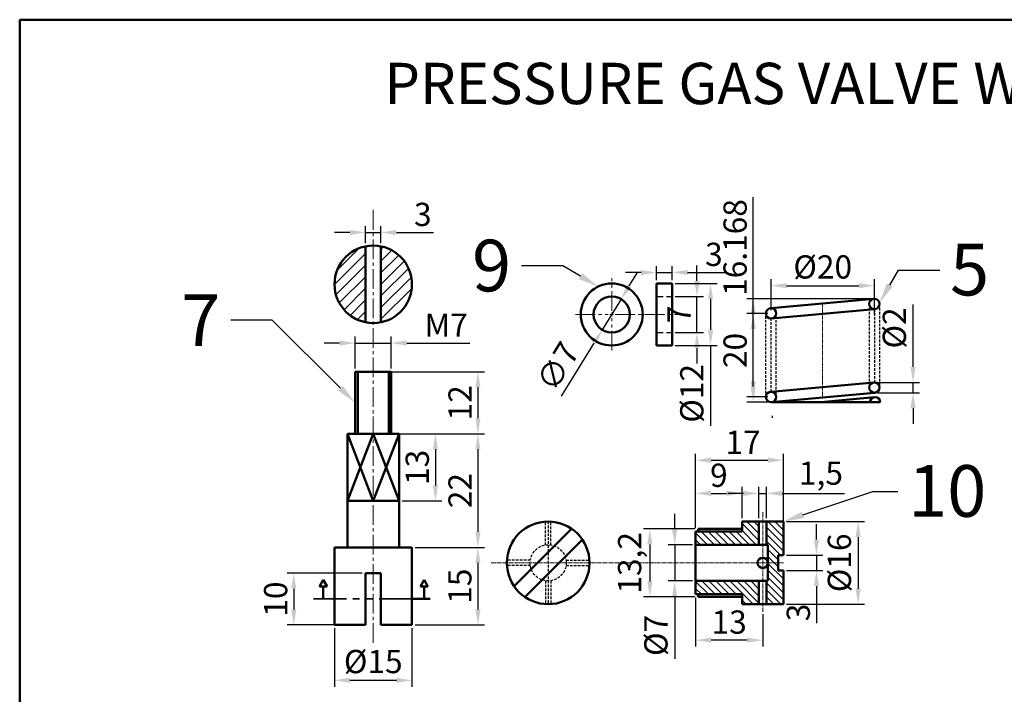
# Model space of a CAD drawing. Units: millimetres. Extents: x 418 to 773, y -46 to 294.
# Tile 5 of 7: x 418 to 609, y 164 to 294. Entities that reach past the tile are written whole.
import ezdxf
from ezdxf import colors
from ezdxf.entities.mleader import LeaderData, LeaderLine
from ezdxf.math import Vec2, Vec3

# ---------------------------------------------------------------- set-up
doc = ezdxf.new("R2010")
doc.units = ezdxf.units.MM
doc.header["$LTSCALE"] = 0.2
for name, pattern in [('CENTER2', [28.575, 19.05, -3.175, 3.175, -3.175]), ('DASHED', [19.05, 12.7, -6.35]), ('PHANTOM', [63.5, 31.75, -6.35, 6.35, -6.35, 6.35, -6.35])]:
    doc.linetypes.add(name, pattern=pattern)
for name, color, linetype, lineweight in [('M-CNTR', 1, 'CENTER2', 18), ('M-DIMS', 2, 'Continuous', 25), ('M-HATC', 8, 'Continuous', 18), ('M-HIDN', 4, 'DASHED', 25), ('M-OUTL', 7, 'Continuous', 50), ('M-SECT', 6, 'PHANTOM', 35), ('M-TEXT', 3, 'Continuous', 25), ('M-TTLB', 7, 'Continuous', 50)]:
    doc.layers.add(name, color=color, linetype=linetype, lineweight=lineweight)
doc.styles.get("Standard").update_dxf_attribs({"font": 'arial.ttf'})
doc.dimstyles.new('ISO-25', dxfattribs={"dimtxt": 4.5, "dimasz": 3, "dimexe": 1.25, "dimexo": 0.625, "dimtad": 1, "dimdec": 1, "dimtxsty": 'Standard', "dimcen": 2.5, "dimadec": 0, "dimazin": 0, "dimtfac": 1, "dimtdec": 1, "dimtmove": 0, "dimatfit": 3, "dimfxl": 1, "dimarcsym": 0})

# ---------------------------------------------------------------- blocks, each defined once
blk = doc.blocks.new('*U1')
at = {"layer": 'M-CNTR', "color": 0, "transparency": 16777216}
blk.add_line((0, -11), (0, 72.91), dxfattribs=at)
blk = doc.blocks.new('*D2')
at = {"layer": 'Defpoints', "color": 0, "transparency": 16777216}
for p in [(489.88, 231.81), (482.88, 226.25), (489.88, 226.25)]:
    blk.add_point(p, dxfattribs=at)
at = {"layer": 'M-DIMS', "color": 0, "lineweight": -2, "transparency": 16777216}
for p, q in [((482.88, 226.88), (482.88, 233.06)), ((489.88, 226.88), (489.88, 233.06)), ((479.88, 231.81), (476.88, 231.81)), ((482.88, 231.81), (489.88, 231.81)), ((492.88, 231.81), (505.11, 231.81))]:
    blk.add_line(p, q, dxfattribs=at)
at = {"layer": 'M-DIMS', "color": 0, "transparency": 16777216}
for points in [[(479.88, 232.31), (479.88, 231.31), (482.88, 231.81)], [(492.88, 232.31), (492.88, 231.31), (489.88, 231.81)]]:
    blk.add_solid(points, dxfattribs=at)
at = {"layer": 'M-DIMS', "color": 0, "transparency": 16777216, "insert": (500.5, 234.69), "char_height": 4.5, "attachment_point": 5}
blk.add_mtext('M7', dxfattribs=at)
blk = doc.blocks.new('*D3')
at = {"layer": 'Defpoints', "color": 0, "transparency": 16777216}
for p in [(487.88, 253.22), (484.88, 250.54), (487.88, 250.54)]:
    blk.add_point(p, dxfattribs=at)
at = {"layer": 'M-DIMS', "color": 0, "lineweight": -2, "transparency": 16777216}
for p, q in [((484.88, 251.16), (484.88, 254.47)), ((487.88, 251.16), (487.88, 254.47)), ((481.88, 253.22), (478.88, 253.22)), ((484.88, 253.22), (487.88, 253.22)), ((490.88, 253.22), (498.08, 253.22))]:
    blk.add_line(p, q, dxfattribs=at)
at = {"layer": 'M-DIMS', "color": 0, "transparency": 16777216}
for points in [[(481.88, 253.72), (481.88, 252.72), (484.88, 253.22)], [(490.88, 253.72), (490.88, 252.72), (487.88, 253.22)]]:
    blk.add_solid(points, dxfattribs=at)
at = {"layer": 'M-DIMS', "color": 0, "transparency": 16777216, "insert": (495.98, 256.14), "char_height": 4.5, "attachment_point": 5}
blk.add_mtext('3', dxfattribs=at)
blk = doc.blocks.new('*D4')
at = {"layer": 'Defpoints', "color": 0, "transparency": 16777216}
for p in [(486.38, 226.25), (486.38, 214.25), (506.65, 214.25)]:
    blk.add_point(p, dxfattribs=at)
at = {"layer": 'M-DIMS', "color": 0, "lineweight": -2, "transparency": 16777216}
for p, q in [((487.01, 226.25), (507.9, 226.25)), ((506.65, 223.25), (506.65, 217.25)), ((487.01, 214.25), (507.9, 214.25))]:
    blk.add_line(p, q, dxfattribs=at)
at = {"layer": 'M-DIMS', "color": 0, "transparency": 16777216}
for points in [[(506.15, 223.25), (507.15, 223.25), (506.65, 226.25)], [(506.15, 217.25), (507.15, 217.25), (506.65, 214.25)]]:
    blk.add_solid(points, dxfattribs=at)
at = {"layer": 'M-DIMS', "color": 0, "transparency": 16777216, "insert": (503.77, 220.25), "char_height": 4.5, "attachment_point": 5, "rotation": 90}
blk.add_mtext('12', dxfattribs=at)
blk = doc.blocks.new('*D5')
at = {"layer": 'Defpoints', "color": 0, "transparency": 16777216}
for p in [(491.38, 214.25), (491.38, 201.25), (498.42, 201.25)]:
    blk.add_point(p, dxfattribs=at)
at = {"layer": 'M-DIMS', "color": 0, "lineweight": -2, "transparency": 16777216}
for p, q in [((492.01, 214.25), (499.67, 214.25)), ((498.42, 211.25), (498.42, 204.25)), ((492.01, 201.25), (499.67, 201.25))]:
    blk.add_line(p, q, dxfattribs=at)
at = {"layer": 'M-DIMS', "color": 0, "transparency": 16777216}
for points in [[(497.92, 211.25), (498.92, 211.25), (498.42, 214.25)], [(497.92, 204.25), (498.92, 204.25), (498.42, 201.25)]]:
    blk.add_solid(points, dxfattribs=at)
at = {"layer": 'M-DIMS', "color": 0, "transparency": 16777216, "insert": (495.49, 207.75), "char_height": 4.5, "attachment_point": 5, "rotation": 90}
blk.add_mtext('13', dxfattribs=at)
blk = doc.blocks.new('*D6')
at = {"layer": 'Defpoints', "color": 0, "transparency": 16777216}
for p in [(503.88, 214.25), (493.88, 192.25), (506.65, 192.25)]:
    blk.add_point(p, dxfattribs=at)
at = {"layer": 'M-DIMS', "color": 0, "lineweight": -2, "transparency": 16777216}
for p, q in [((504.5, 214.25), (507.9, 214.25)), ((506.65, 211.25), (506.65, 195.25)), ((494.51, 192.25), (507.9, 192.25))]:
    blk.add_line(p, q, dxfattribs=at)
at = {"layer": 'M-DIMS', "color": 0, "transparency": 16777216}
for points in [[(506.15, 211.25), (507.15, 211.25), (506.65, 214.25)], [(506.15, 195.25), (507.15, 195.25), (506.65, 192.25)]]:
    blk.add_solid(points, dxfattribs=at)
at = {"layer": 'M-DIMS', "color": 0, "transparency": 16777216, "insert": (503.77, 203.25), "char_height": 4.5, "attachment_point": 5, "rotation": 90}
blk.add_mtext('22', dxfattribs=at)
blk = doc.blocks.new('*D7')
at = {"layer": 'Defpoints', "color": 0, "transparency": 16777216}
for p in [(493.88, 192.25), (493.88, 177.25), (506.65, 177.25)]:
    blk.add_point(p, dxfattribs=at)
at = {"layer": 'M-DIMS', "color": 0, "lineweight": -2, "transparency": 16777216}
for p, q in [((494.51, 192.25), (507.9, 192.25)), ((506.65, 189.25), (506.65, 180.25)), ((494.51, 177.25), (507.9, 177.25))]:
    blk.add_line(p, q, dxfattribs=at)
at = {"layer": 'M-DIMS', "color": 0, "transparency": 16777216}
for points in [[(506.15, 189.25), (507.15, 189.25), (506.65, 192.25)], [(506.15, 180.25), (507.15, 180.25), (506.65, 177.25)]]:
    blk.add_solid(points, dxfattribs=at)
at = {"layer": 'M-DIMS', "color": 0, "transparency": 16777216, "insert": (503.73, 184.75), "char_height": 4.5, "attachment_point": 5, "rotation": 90}
blk.add_mtext('15', dxfattribs=at)
blk = doc.blocks.new('*D8')
at = {"layer": 'Defpoints', "color": 0, "transparency": 16777216}
for p in [(478.88, 177.25), (493.88, 177.25), (493.88, 166.53)]:
    blk.add_point(p, dxfattribs=at)
at = {"layer": 'M-DIMS', "color": 0, "lineweight": -2, "transparency": 16777216}
for p, q in [((478.88, 176.63), (478.88, 165.28)), ((493.88, 176.63), (493.88, 165.28)), ((481.88, 166.53), (490.88, 166.53))]:
    blk.add_line(p, q, dxfattribs=at)
at = {"layer": 'M-DIMS', "color": 0, "transparency": 16777216}
for points in [[(481.88, 167.03), (481.88, 166.03), (478.88, 166.53)], [(490.88, 167.03), (490.88, 166.03), (493.88, 166.53)]]:
    blk.add_solid(points, dxfattribs=at)
at = {"layer": 'M-DIMS', "color": 0, "transparency": 16777216, "insert": (486.38, 169.58), "char_height": 4.5, "attachment_point": 5}
blk.add_mtext('%%C15', dxfattribs=at)
blk = doc.blocks.new('*D9')
at = {"layer": 'Defpoints', "color": 0, "transparency": 16777216}
for p in [(484.88, 187.25), (471, 177.25), (484.88, 177.25)]:
    blk.add_point(p, dxfattribs=at)
at = {"layer": 'M-DIMS', "color": 0, "lineweight": -2, "transparency": 16777216}
for p, q in [((484.26, 187.25), (469.75, 187.25)), ((471, 184.25), (471, 180.25)), ((484.26, 177.25), (469.75, 177.25))]:
    blk.add_line(p, q, dxfattribs=at)
at = {"layer": 'M-DIMS', "color": 0, "transparency": 16777216}
for points in [[(470.5, 184.25), (471.5, 184.25), (471, 187.25)], [(470.5, 180.25), (471.5, 180.25), (471, 177.25)]]:
    blk.add_solid(points, dxfattribs=at)
at = {"layer": 'M-DIMS', "color": 0, "transparency": 16777216, "insert": (468.07, 182.25), "char_height": 4.5, "attachment_point": 5, "rotation": 90}
blk.add_mtext('10', dxfattribs=at)
blk = doc.blocks.new('*U10')
at = {"layer": 'M-CNTR', "color": 0, "transparency": 16777216}
for p, q in [((0, 0.7), (0, 7)), ((-7, 0), (-0.7, 0)), ((0.7, 0), (13.95, 0)), ((0, -7), (0, -0.7))]:
    blk.add_line(p, q, dxfattribs=at)
at = {"layer": 'M-CNTR', "color": 0, "linetype": 'Continuous', "transparency": 16777216}
for p, q in [((-0.35, 0), (0.35, 0)), ((0, -0.35), (0, 0.35))]:
    blk.add_line(p, q, dxfattribs=at)
blk = doc.blocks.new('*D11')
at = {"layer": 'Defpoints', "color": 0, "ltscale": 0.2, "transparency": 16777216}
for p in [(544.23, 245.48), (541.23, 243.35), (544.23, 243.35)]:
    blk.add_point(p, dxfattribs=at)
at = {"layer": 'M-DIMS', "color": 0, "lineweight": -2, "ltscale": 0.2, "transparency": 16777216}
for p, q in [((541.23, 243.98), (541.23, 246.73)), ((544.23, 243.98), (544.23, 246.73)), ((538.23, 245.48), (535.23, 245.48)), ((541.23, 245.48), (544.23, 245.48)), ((547.23, 245.48), (554.43, 245.48))]:
    blk.add_line(p, q, dxfattribs=at)
at = {"layer": 'M-DIMS', "color": 0, "ltscale": 0.2, "transparency": 16777216}
for points in [[(538.23, 245.98), (538.23, 244.98), (541.23, 245.48)], [(547.23, 245.98), (547.23, 244.98), (544.23, 245.48)]]:
    blk.add_solid(points, dxfattribs=at)
at = {"layer": 'M-DIMS', "color": 0, "ltscale": 0.2, "transparency": 16777216, "insert": (552.33, 248.4), "char_height": 4.5, "attachment_point": 5}
blk.add_mtext('3', dxfattribs=at)
blk = doc.blocks.new('*D12')
at = {"layer": 'Defpoints', "color": 0, "ltscale": 0.2, "transparency": 16777216}
for p in [(544.23, 243.35), (544.23, 231.35), (551.69, 231.35)]:
    blk.add_point(p, dxfattribs=at)
at = {"layer": 'M-DIMS', "color": 0, "lineweight": -2, "ltscale": 0.2, "transparency": 16777216}
for p, q in [((544.86, 243.35), (552.94, 243.35)), ((551.69, 240.35), (551.69, 234.35)), ((544.86, 231.35), (552.94, 231.35)), ((551.69, 231.35), (551.69, 215.81))]:
    blk.add_line(p, q, dxfattribs=at)
at = {"layer": 'M-DIMS', "color": 0, "ltscale": 0.2, "transparency": 16777216}
for points in [[(551.19, 240.35), (552.19, 240.35), (551.69, 243.35)], [(551.19, 234.35), (552.19, 234.35), (551.69, 231.35)]]:
    blk.add_solid(points, dxfattribs=at)
at = {"layer": 'M-DIMS', "color": 0, "ltscale": 0.2, "transparency": 16777216, "insert": (548.64, 222.08), "char_height": 4.5, "attachment_point": 5, "rotation": 90}
blk.add_mtext('%%C12', dxfattribs=at)
blk = doc.blocks.new('*D13')
at = {"layer": 'Defpoints', "color": 0, "ltscale": 0.2, "transparency": 16777216}
for p in [(534.38, 240.33), (530.72, 234.37)]:
    blk.add_point(p, dxfattribs=at)
at = {"layer": 'M-DIMS', "color": 0, "lineweight": -2, "ltscale": 0.2, "transparency": 16777216}
for p, q in [((535.95, 242.89), (537.52, 245.45)), ((534.38, 240.33), (530.72, 234.37)), ((522.81, 221.51), (529.15, 231.81))]:
    blk.add_line(p, q, dxfattribs=at)
at = {"layer": 'M-DIMS', "color": 0, "ltscale": 0.2, "transparency": 16777216}
for points in [[(535.53, 243.15), (536.38, 242.63), (534.38, 240.33)], [(528.72, 232.08), (529.57, 231.55), (530.72, 234.37)]]:
    blk.add_solid(points, dxfattribs=at)
at = {"layer": 'M-DIMS', "color": 0, "ltscale": 0.2, "transparency": 16777216, "insert": (522.6, 226.98), "char_height": 4.5, "attachment_point": 5, "rotation": 58.4274}
blk.add_mtext('∅7', dxfattribs=at)
blk = doc.blocks.new('*D14')
at = {"layer": 'Defpoints', "color": 0, "ltscale": 0.2, "transparency": 16777216}
for p in [(565.79, 209.14), (548.79, 195.35), (565.79, 195.35)]:
    blk.add_point(p, dxfattribs=at)
at = {"layer": 'M-DIMS', "color": 0, "lineweight": -2, "ltscale": 0.2, "transparency": 16777216}
for p, q in [((548.79, 195.97), (548.79, 210.39)), ((565.79, 195.97), (565.79, 210.39)), ((551.79, 209.14), (562.79, 209.14))]:
    blk.add_line(p, q, dxfattribs=at)
at = {"layer": 'M-DIMS', "color": 0, "ltscale": 0.2, "transparency": 16777216}
for points in [[(551.79, 209.64), (551.79, 208.64), (548.79, 209.14)], [(562.79, 209.64), (562.79, 208.64), (565.79, 209.14)]]:
    blk.add_solid(points, dxfattribs=at)
at = {"layer": 'M-DIMS', "color": 0, "ltscale": 0.2, "transparency": 16777216, "insert": (557.97, 212.02), "char_height": 4.5, "attachment_point": 5}
blk.add_mtext('17', dxfattribs=at)
blk = doc.blocks.new('*D15')
at = {"layer": 'Defpoints', "color": 0, "ltscale": 0.2, "transparency": 16777216}
for p in [(557.79, 202.72), (548.79, 198.4), (557.79, 197.27)]:
    blk.add_point(p, dxfattribs=at)
at = {"layer": 'M-DIMS', "color": 0, "lineweight": -2, "ltscale": 0.2, "transparency": 16777216}
for p, q in [((548.79, 199.02), (548.79, 203.97)), ((557.79, 197.89), (557.79, 203.97)), ((551.79, 202.72), (554.79, 202.72))]:
    blk.add_line(p, q, dxfattribs=at)
at = {"layer": 'M-DIMS', "color": 0, "ltscale": 0.2, "transparency": 16777216}
for points in [[(551.79, 203.22), (551.79, 202.22), (548.79, 202.72)], [(554.79, 203.22), (554.79, 202.22), (557.79, 202.72)]]:
    blk.add_solid(points, dxfattribs=at)
at = {"layer": 'M-DIMS', "color": 0, "ltscale": 0.2, "transparency": 16777216, "insert": (553.29, 205.64), "char_height": 4.5, "attachment_point": 5}
blk.add_mtext('9', dxfattribs=at)
blk = doc.blocks.new('*D16')
at = {"layer": 'Defpoints', "color": 0, "ltscale": 0.2, "transparency": 16777216}
for p in [(562.54, 202.72), (561.04, 197.27), (562.54, 197.27)]:
    blk.add_point(p, dxfattribs=at)
at = {"layer": 'M-DIMS', "color": 0, "lineweight": -2, "ltscale": 0.2, "transparency": 16777216}
for p, q in [((561.04, 197.89), (561.04, 203.97)), ((562.54, 197.89), (562.54, 203.97)), ((558.04, 202.72), (555.04, 202.72)), ((561.04, 202.72), (562.54, 202.72)), ((565.54, 202.72), (577.59, 202.72))]:
    blk.add_line(p, q, dxfattribs=at)
at = {"layer": 'M-DIMS', "color": 0, "ltscale": 0.2, "transparency": 16777216}
for points in [[(558.04, 203.22), (558.04, 202.22), (561.04, 202.72)], [(565.54, 203.22), (565.54, 202.22), (562.54, 202.72)]]:
    blk.add_solid(points, dxfattribs=at)
at = {"layer": 'M-DIMS', "color": 0, "ltscale": 0.2, "transparency": 16777216, "insert": (573.06, 206.05), "char_height": 4.5, "attachment_point": 5}
blk.add_mtext('1,5', dxfattribs=at)
blk = doc.blocks.new('*D17')
at = {"layer": 'Defpoints', "color": 0, "ltscale": 0.2, "transparency": 16777216}
for p in [(565.79, 190.77), (565.79, 187.77), (572.19, 187.77)]:
    blk.add_point(p, dxfattribs=at)
at = {"layer": 'M-DIMS', "color": 0, "lineweight": -2, "ltscale": 0.2, "transparency": 16777216}
for p, q in [((572.19, 193.77), (572.19, 196.77)), ((566.41, 190.77), (573.44, 190.77)), ((572.19, 190.77), (572.19, 187.77)), ((566.41, 187.77), (573.44, 187.77)), ((572.19, 184.77), (572.19, 177.57))]:
    blk.add_line(p, q, dxfattribs=at)
at = {"layer": 'M-DIMS', "color": 0, "ltscale": 0.2, "transparency": 16777216}
for points in [[(571.69, 193.77), (572.69, 193.77), (572.19, 190.77)], [(571.69, 184.77), (572.69, 184.77), (572.19, 187.77)]]:
    blk.add_solid(points, dxfattribs=at)
at = {"layer": 'M-DIMS', "color": 0, "ltscale": 0.2, "transparency": 16777216, "insert": (569.26, 179.67), "char_height": 4.5, "attachment_point": 5, "rotation": 90}
blk.add_mtext('3', dxfattribs=at)
blk = doc.blocks.new('*D18')
at = {"layer": 'Defpoints', "color": 0, "ltscale": 0.2, "transparency": 16777216}
for p in [(565.79, 197.27), (565.79, 181.27), (580.26, 181.27)]:
    blk.add_point(p, dxfattribs=at)
at = {"layer": 'M-DIMS', "color": 0, "lineweight": -2, "ltscale": 0.2, "transparency": 16777216}
for p, q in [((566.41, 197.27), (581.51, 197.27)), ((580.26, 194.27), (580.26, 184.27)), ((566.41, 181.27), (581.51, 181.27))]:
    blk.add_line(p, q, dxfattribs=at)
at = {"layer": 'M-DIMS', "color": 0, "ltscale": 0.2, "transparency": 16777216}
for points in [[(579.76, 194.27), (580.76, 194.27), (580.26, 197.27)], [(579.76, 184.27), (580.76, 184.27), (580.26, 181.27)]]:
    blk.add_solid(points, dxfattribs=at)
at = {"layer": 'M-DIMS', "color": 0, "ltscale": 0.2, "transparency": 16777216, "insert": (577.21, 189.27), "char_height": 4.5, "attachment_point": 5, "rotation": 90}
blk.add_mtext('%%C16', dxfattribs=at)
blk = doc.blocks.new('*D19')
at = {"layer": 'Defpoints', "color": 0, "ltscale": 0.2, "transparency": 16777216}
for p in [(548.79, 183.19), (561.79, 179.97), (548.79, 174.3)]:
    blk.add_point(p, dxfattribs=at)
at = {"layer": 'M-DIMS', "color": 0, "lineweight": -2, "ltscale": 0.2, "transparency": 16777216}
for p, q in [((548.79, 182.56), (548.79, 173.05)), ((561.79, 179.34), (561.79, 173.05)), ((558.79, 174.3), (551.79, 174.3))]:
    blk.add_line(p, q, dxfattribs=at)
at = {"layer": 'M-DIMS', "color": 0, "ltscale": 0.2, "transparency": 16777216}
for points in [[(551.79, 174.8), (551.79, 173.8), (548.79, 174.3)], [(558.79, 174.8), (558.79, 173.8), (561.79, 174.3)]]:
    blk.add_solid(points, dxfattribs=at)
at = {"layer": 'M-DIMS', "color": 0, "ltscale": 0.2, "transparency": 16777216, "insert": (555.29, 177.22), "char_height": 4.5, "attachment_point": 5}
blk.add_mtext('13', dxfattribs=at)
blk = doc.blocks.new('*D20')
at = {"layer": 'Defpoints', "color": 0, "ltscale": 0.2, "transparency": 16777216}
for p in [(548.79, 192.77), (544.74, 185.77), (548.79, 185.77)]:
    blk.add_point(p, dxfattribs=at)
at = {"layer": 'M-DIMS', "color": 0, "lineweight": -2, "ltscale": 0.2, "transparency": 16777216}
for p, q in [((544.74, 195.77), (544.74, 198.77)), ((548.16, 192.77), (543.49, 192.77)), ((544.74, 192.77), (544.74, 185.77)), ((548.16, 185.77), (543.49, 185.77)), ((544.74, 182.77), (544.74, 170.67))]:
    blk.add_line(p, q, dxfattribs=at)
at = {"layer": 'M-DIMS', "color": 0, "ltscale": 0.2, "transparency": 16777216}
for points in [[(544.24, 195.77), (545.24, 195.77), (544.74, 192.77)], [(544.24, 182.77), (545.24, 182.77), (544.74, 185.77)]]:
    blk.add_solid(points, dxfattribs=at)
at = {"layer": 'M-DIMS', "color": 0, "ltscale": 0.2, "transparency": 16777216, "insert": (541.69, 175.22), "char_height": 4.5, "attachment_point": 5, "rotation": 90}
blk.add_mtext('%%C7', dxfattribs=at)
blk = doc.blocks.new('*D21')
at = {"layer": 'Defpoints', "color": 0, "ltscale": 0.2, "transparency": 16777216}
for p in [(549.29, 195.85), (539.93, 182.69), (549.29, 182.69)]:
    blk.add_point(p, dxfattribs=at)
at = {"layer": 'M-DIMS', "color": 0, "lineweight": -2, "ltscale": 0.2, "transparency": 16777216}
for p, q in [((548.66, 195.85), (538.68, 195.85)), ((539.93, 192.85), (539.93, 185.69)), ((548.66, 182.69), (538.68, 182.69))]:
    blk.add_line(p, q, dxfattribs=at)
at = {"layer": 'M-DIMS', "color": 0, "ltscale": 0.2, "transparency": 16777216}
for points in [[(539.43, 192.85), (540.43, 192.85), (539.93, 195.85)], [(539.43, 185.69), (540.43, 185.69), (539.93, 182.69)]]:
    blk.add_solid(points, dxfattribs=at)
at = {"layer": 'M-DIMS', "color": 0, "ltscale": 0.2, "transparency": 16777216, "insert": (536.6, 189.27), "char_height": 4.5, "attachment_point": 5, "rotation": 90}
blk.add_mtext('13,2', dxfattribs=at)
blk = doc.blocks.new('*D41')
at = {"layer": 'Defpoints', "color": 0, "ltscale": 0.2, "transparency": 16777216}
for p in [(583.4, 242.92), (563.4, 237.55), (583.4, 236.84)]:
    blk.add_point(p, dxfattribs=at)
at = {"layer": 'M-DIMS', "color": 0, "lineweight": -2, "ltscale": 0.2, "transparency": 16777216}
for p, q in [((563.4, 238.18), (563.4, 244.17)), ((583.4, 237.46), (583.4, 244.17)), ((566.4, 242.92), (580.4, 242.92))]:
    blk.add_line(p, q, dxfattribs=at)
at = {"layer": 'M-DIMS', "color": 0, "ltscale": 0.2, "transparency": 16777216}
for points in [[(566.4, 243.42), (566.4, 242.42), (563.4, 242.92)], [(580.4, 243.42), (580.4, 242.42), (583.4, 242.92)]]:
    blk.add_solid(points, dxfattribs=at)
at = {"layer": 'M-DIMS', "color": 0, "ltscale": 0.2, "transparency": 16777216, "insert": (573.4, 245.97), "char_height": 4.5, "attachment_point": 5}
blk.add_mtext('%%C20', dxfattribs=at)
blk = doc.blocks.new('*D42')
at = {"layer": 'Defpoints', "color": 0, "ltscale": 0.2, "transparency": 16777216}
for p in [(583.4, 224.21), (583.4, 222.21), (590.89, 222.21)]:
    blk.add_point(p, dxfattribs=at)
at = {"layer": 'M-DIMS', "color": 0, "lineweight": -2, "ltscale": 0.2, "transparency": 16777216}
for p, q in [((590.89, 227.21), (590.89, 239.26)), ((584.02, 224.21), (592.14, 224.21)), ((590.89, 222.21), (590.89, 224.21)), ((584.02, 222.21), (592.14, 222.21)), ((590.89, 219.21), (590.89, 216.21))]:
    blk.add_line(p, q, dxfattribs=at)
at = {"layer": 'M-DIMS', "color": 0, "ltscale": 0.2, "transparency": 16777216}
for points in [[(590.39, 227.21), (591.39, 227.21), (590.89, 224.21)], [(590.39, 219.21), (591.39, 219.21), (590.89, 222.21)]]:
    blk.add_solid(points, dxfattribs=at)
at = {"layer": 'M-DIMS', "color": 0, "ltscale": 0.2, "transparency": 16777216, "insert": (587.85, 234.74), "char_height": 4.5, "attachment_point": 5, "rotation": 90}
blk.add_mtext('%%C2', dxfattribs=at)
blk = doc.blocks.new('*D96')
at = {"layer": 'Defpoints', "color": 0, "ltscale": 0.2, "transparency": 16777216}
for p in [(544.23443, 240.852643), (549.050173, 240.852643), (544.23443, 233.852643)]:
    blk.add_point(p, dxfattribs=at)
at = {"layer": 'M-DIMS', "color": 0, "lineweight": -2, "ltscale": 0.2, "transparency": 16777216}
for p, q in [((549.050173, 243.852643), (549.050173, 246.852643)), ((544.85943, 240.852643), (550.300173, 240.852643)), ((549.050173, 233.852643), (549.050173, 240.852643)), ((544.85943, 233.852643), (550.300173, 233.852643)), ((549.050173, 230.852643), (549.050173, 227.852643))]:
    blk.add_line(p, q, dxfattribs=at)
at = {"layer": 'M-DIMS', "color": 0, "ltscale": 0.2, "transparency": 16777216}
for points in [[(548.550173, 243.852643), (549.550173, 243.852643), (549.050173, 240.852643)], [(548.550173, 230.852643), (549.550173, 230.852643), (549.050173, 233.852643)]]:
    blk.add_solid(points, dxfattribs=at)
at = {"layer": 'M-DIMS', "color": 0, "ltscale": 0.2, "transparency": 16777216, "insert": (546.175173, 237.352643), "char_height": 4.5, "attachment_point": 5, "rotation": 90}
blk.add_mtext('7', dxfattribs=at)
blk = doc.blocks.new('*D97')
at = {"layer": 'Defpoints', "color": 0, "ltscale": 0.2, "transparency": 16777216}
for p in [(559.94, 240.38), (583.4, 240.38), (563.4, 220.38)]:
    blk.add_point(p, dxfattribs=at)
at = {"layer": 'M-DIMS', "color": 0, "lineweight": -2, "ltscale": 0.2, "transparency": 16777216}
for p, q in [((582.77, 240.38), (558.69, 240.38)), ((559.94, 223.38), (559.94, 237.38)), ((562.77, 220.38), (558.69, 220.38))]:
    blk.add_line(p, q, dxfattribs=at)
at = {"layer": 'M-DIMS', "color": 0, "ltscale": 0.2, "transparency": 16777216}
for points in [[(559.44, 237.38), (560.44, 237.38), (559.94, 240.38)], [(559.44, 223.38), (560.44, 223.38), (559.94, 220.38)]]:
    blk.add_solid(points, dxfattribs=at)
at = {"layer": 'M-DIMS', "color": 0, "ltscale": 0.2, "transparency": 16777216, "insert": (557.02, 230.38), "char_height": 4.5, "attachment_point": 5, "rotation": 90}
blk.add_mtext('20', dxfattribs=at)
blk = doc.blocks.new('*D98')
at = {"layer": 'Defpoints', "color": 0, "ltscale": 0.2, "transparency": 16777216}
for p in [(559.94, 237.55), (563.4, 237.55), (563.4, 221.38)]:
    blk.add_point(p, dxfattribs=at)
at = {"layer": 'M-DIMS', "color": 0, "lineweight": -2, "ltscale": 0.2, "transparency": 16777216}
for p, q in [((559.94, 237.55), (559.94, 260.07)), ((562.77, 237.55), (558.69, 237.55)), ((559.94, 224.38), (559.94, 234.55)), ((562.77, 221.38), (558.69, 221.38))]:
    blk.add_line(p, q, dxfattribs=at)
at = {"layer": 'M-DIMS', "color": 0, "ltscale": 0.2, "transparency": 16777216}
for points in [[(559.44, 234.55), (560.44, 234.55), (559.94, 237.55)], [(559.44, 224.38), (560.44, 224.38), (559.94, 221.38)]]:
    blk.add_solid(points, dxfattribs=at)
at = {"layer": 'M-DIMS', "color": 0, "ltscale": 0.2, "transparency": 16777216, "insert": (557.02, 250.31), "char_height": 4.5, "attachment_point": 5, "rotation": 90}
blk.add_mtext('16.168', dxfattribs=at)

msp = doc.modelspace()

# ---------------------------------------------------------------- hatches: boundary and pattern name
at = {"layer": 'M-HATC'}
h = msp.add_hatch(dxfattribs=at)
h.set_pattern_fill('ANSI31', color=256, scale=0.5)
h.paths.add_polyline_path([(493.8841, 243.1886, 0.35639396), (487.8841, 250.5371), (487.8841, 235.8401, 0.35639396)])
h.paths.add_polyline_path([(484.8841, 250.5371, 0.35639396), (478.8841, 243.1886, 0.35639396), (484.8841, 235.8401)])
at = {"layer": 'M-HATC', "ltscale": 0.2}
h = msp.add_hatch(dxfattribs=at)
h.set_pattern_fill('ANSI31', color=256, scale=0.3, angle=90)
h.set_pattern_definition([(135, (-26.4443, -19.0433), (-0.6735192, -0.6735192), [])])
h.paths.add_polyline_path([(561.0383, 197.2675), (557.7883, 197.2675), (557.7883, 195.3475), (548.7883, 195.3475), (548.7883, 192.7675), (561.0383, 192.7675)])
h.paths.add_polyline_path([(565.7883, 197.2675), (562.5383, 197.2675), (562.5383, 192.7675), (562.7883, 192.7675), (562.7883, 189.2675), (564.7883, 189.2675), (564.7883, 190.7675), (565.7883, 190.7675)])
h.paths.add_polyline_path([(561.0383, 185.7675), (548.7883, 185.7675), (548.7883, 183.1875), (557.7883, 183.1875), (557.7883, 181.2675), (561.0383, 181.2675)])
h.paths.add_polyline_path([(565.7883, 187.7675), (564.7883, 187.7675), (564.7883, 189.2675), (562.7883, 189.2675), (562.7883, 185.7675), (562.5383, 185.7675), (562.5383, 181.2675), (565.7883, 181.2675)])

# ---------------------------------------------------------------- linework, layer by layer
at = {"layer": 'M-CNTR', "ltscale": 0.2}
for p, q in [((573.352, 239.4644), (573.352, 221.2904)), ((561.7883, 179.8039), (561.7883, 199.1506)), ((509.1945, 189.2675), (565.7883, 189.2675))]:
    msp.add_line(p, q, dxfattribs=at)
at = {"layer": 'M-HIDN', "ltscale": 0.5}
for p, q in [((541.2344, 240.8526), (544.2344, 240.8526)), ((541.2344, 233.8526), (544.2344, 233.8526))]:
    msp.add_line(p, q, dxfattribs=at)
at = {"layer": 'M-HIDN', "ltscale": 0.2}
for p, q in [((582.3975, 239.3784), (582.3975, 223.2107)), ((583.3975, 238.3784), (583.3975, 224.2107)), ((584.3975, 239.3784), (584.3975, 223.2107)), ((562.3975, 221.2912), (562.3975, 237.6417)), ((563.3975, 222.3868), (563.3975, 236.5461)), ((564.3975, 221.2912), (564.4017, 237.5503)), ((519.7538, 192.7316), (519.7538, 197.2675)), ((520.2538, 197.2675), (520.2538, 181.2675)), ((520.7538, 192.7316), (520.7538, 197.2675)), ((516.7897, 189.7675), (512.2538, 189.7675)), ((516.7897, 188.7675), (512.2538, 188.7675)), ((523.7179, 189.7675), (528.2538, 189.7675)), ((523.7179, 188.7675), (528.2538, 188.7675)), ((519.7538, 185.8034), (519.7538, 181.2675)), ((520.7538, 185.8034), (520.7538, 181.2675))]:
    msp.add_line(p, q, dxfattribs=at)
msp.add_circle((520.2538, 189.2675), 3.5, dxfattribs=at)
at = {"layer": 'M-OUTL'}
for p, q in [((484.8841, 235.8401), (484.8841, 250.5371)), ((487.8841, 235.8401), (487.8841, 250.5371)), ((486.3841, 226.254), (482.8841, 226.254)), ((482.8841, 226.254), (482.8841, 214.254)), ((483.3841, 226.254), (483.3841, 214.254)), ((489.8841, 226.254), (486.3841, 226.254)), ((489.3841, 214.254), (489.3841, 226.254)), ((489.8841, 214.254), (489.8841, 226.254)), ((481.3841, 201.254), (481.3841, 214.254)), ((481.3841, 214.254), (482.8841, 214.254)), ((481.3841, 214.254), (486.3841, 201.254)), ((481.3841, 201.254), (486.3841, 214.254)), ((482.8841, 214.254), (489.8841, 214.254)), ((486.3841, 214.254), (491.3841, 214.254)), ((486.3841, 201.254), (491.3841, 214.254)), ((486.3841, 214.254), (491.3841, 201.254)), ((491.3841, 214.254), (491.3841, 201.254)), ((491.3841, 201.254), (481.3841, 201.254)), ((481.3841, 201.254), (481.3841, 192.254)), ((491.3841, 201.254), (491.3841, 192.254)), ((493.8841, 192.254), (478.8841, 192.254)), ((478.8841, 192.254), (478.8841, 177.254)), ((493.8841, 177.254), (493.8841, 192.254)), ((484.8841, 177.254), (484.8841, 187.254)), ((484.8841, 187.254), (487.8841, 187.254)), ((487.8841, 187.254), (487.8841, 177.254)), ((476.7153, 185.9812), (475.9804, 184.7084)), ((476.7153, 185.9812), (477.4501, 184.7084)), ((496.2443, 185.9812), (495.5094, 184.7084)), ((496.2443, 185.9812), (496.9791, 184.7084)), ((475.9804, 184.7084), (477.4501, 184.7084)), ((476.7153, 182.3216), (476.7153, 184.7084)), ((495.5094, 184.7084), (496.9791, 184.7084)), ((496.2443, 182.3216), (496.2443, 184.7084)), ((493.8841, 182.3216), (497.4174, 182.3216)), ((478.8841, 177.254), (484.8841, 177.254)), ((487.8841, 177.254), (493.8841, 177.254))]:
    msp.add_line(p, q, dxfattribs=at)
at = {"layer": 'M-OUTL', "ltscale": 0.5}
for p, q in [((541.2344, 243.3526), (541.2344, 231.3526)), ((544.2344, 243.3526), (541.2344, 243.3526)), ((544.2344, 231.3526), (544.2344, 243.3526)), ((541.2344, 231.3526), (544.2344, 231.3526))]:
    msp.add_line(p, q, dxfattribs=at)
at = {"layer": 'M-OUTL', "ltscale": 0.2}
for p, q in [((563.3975, 238.5544), (583.3065, 240.3743)), ((563.3975, 236.5461), (583.3975, 238.3784)), ((563.3975, 222.3868), (583.3065, 224.2066)), ((563.3975, 220.3784), (583.3975, 222.2107)), ((573.0331, 220.3951), (583.4546, 221.3477)), ((563.58, 220.3951), (584.5447, 220.3951)), ((557.7883, 197.2675), (565.7883, 197.2675)), ((557.7883, 195.3475), (557.7883, 197.2675)), ((561.0383, 192.7675), (561.0383, 197.2675)), ((562.5383, 192.7675), (562.5383, 197.2675)), ((565.7883, 197.2675), (565.7883, 190.7675)), ((524.7497, 195.8847), (513.6366, 184.7717)), ((548.7883, 183.1875), (548.7883, 195.3475)), ((548.7883, 195.3475), (557.7883, 195.3475)), ((549.2883, 195.8475), (557.7883, 195.8475)), ((549.2883, 195.3475), (549.2883, 195.8475)), ((526.871, 193.7634), (515.7579, 182.6503)), ((548.7883, 192.7675), (562.7883, 192.7675)), ((562.7883, 192.7675), (562.7883, 185.7675)), ((565.7883, 190.7675), (564.7883, 190.7675)), ((564.7883, 190.7675), (564.7883, 187.7675)), ((564.7883, 187.7675), (565.7883, 187.7675)), ((565.7883, 187.7675), (565.7883, 181.2675)), ((562.7883, 185.7675), (548.7883, 185.7675)), ((561.0383, 181.2675), (561.0383, 185.7675)), ((562.5383, 181.2675), (562.5383, 185.7675)), ((548.7883, 183.1875), (557.7883, 183.1875)), ((549.2883, 183.1875), (549.2883, 182.6875)), ((557.7883, 181.2675), (557.7883, 183.1875)), ((549.2883, 182.6875), (557.7883, 182.6875)), ((565.7883, 181.2675), (557.7883, 181.2675))]:
    msp.add_line(p, q, dxfattribs=at)
at = {"layer": 'M-OUTL'}
msp.add_circle((486.3841, 243.1886), 7.5, dxfattribs=at)
at = {"layer": 'M-OUTL', "ltscale": 0.5}
for radius in [6, 3.5]:
    msp.add_circle((532.5491, 237.3526), radius, dxfattribs=at)
at = {"layer": 'M-OUTL', "ltscale": 0.2}
for centre, radius in [((583.3975, 239.3784), 1), ((563.3975, 237.5503), 1.0042), ((583.3975, 223.2107), 1), ((563.3975, 221.3826), 1.0042), ((520.2538, 189.2675), 8), ((561.7883, 189.2675), 1)]:
    msp.add_circle(centre, radius, dxfattribs=at)
for centre, radius, start, end in [((583.5457, 220.3519), 1, 2.478537, 177.521463), ((563.5457, 218.5238), 1.0042, 270, 280.469169)]:
    msp.add_arc(centre, radius, start, end, dxfattribs=at)
at = {"layer": 'M-SECT'}
msp.add_line((493.8841, 182.3216), (474.5465, 182.3216), dxfattribs=at)
at = {"layer": 'M-TTLB', "ltscale": 0.2}
msp.add_lwpolyline([(417.9371, 294.4119), (773.2687, 294.4119), (773.2687, -46.4726), (417.9371, -46.4726)], close=True, dxfattribs=at)

# ---------------------------------------------------------------- block references
at = {"layer": 'M-CNTR'}
for name, p in [('*U1', (486.3841, 184.754)), ('*U10', (532.5491, 237.3526))]:
    msp.add_blockref(name, p, dxfattribs=at)

# ---------------------------------------------------------------- texts
at = {"layer": 'M-TEXT', "ltscale": 0.2, "insert": (483.7429, 286.0654), "char_height": 8, "attachment_point": 1}
msp.add_mtext_dynamic_manual_height_columns('\\pxqc;PRESSURE GAS VALVE WITH SAFETY DEVICE', width=230.482278, gutter_width=12.5, heights=[0], dxfattribs=at)

# ---------------------------------------------------------------- dimensions: what is measured, and where the dimension line sits
at = {"layer": 'M-DIMS', "ltscale": 0.2}
for base, p1, p2, override, picture, middle in [((559.9433, 237.5503), (563.3975, 221.3826), (563.3975, 237.5503), {"dimdec": 3, "dimlfac": 1, "dimrnd": 0, "dimzin": 0, "dimdsep": 46, "dimlunit": 2}, '*D98', (557.0208, 250.3088)), ((549.0502, 240.8526), (544.2344, 233.8526), (544.2344, 240.8526), {"dimdec": 0, "dimlfac": 1, "dimrnd": 0, "dimzin": 0, "dimdsep": 46, "dimlunit": 2}, '*D96', (546.1752, 237.3526)), ((559.9433, 240.3784), (563.3975, 220.3784), (583.3975, 240.3784), {"dimdec": 0, "dimlfac": 1, "dimrnd": 0, "dimzin": 0, "dimdsep": 46, "dimlunit": 2}, '*D97', (557.0208, 230.3784)), ((572.1854, 187.7675), (565.7883, 190.7675), (565.7883, 187.7675), {"dimclrd": 0, "dimclre": 0, "dimclrt": 0}, '*D17', (569.2613, 179.6691)), ((539.9324, 182.6875), (549.2883, 195.8475), (549.2883, 182.6875), {"dimclrd": 0, "dimclre": 0, "dimclrt": 0}, '*D21', (536.6031, 189.2675))]:
    dim = msp.add_linear_dim(base=base, p1=p1, p2=p2, angle=90, dimstyle='ISO-25', override=override, dxfattribs=at)
    dim.commit()
    dim.dimension.update_dxf_attribs({"geometry": picture, "text_midpoint": middle})
at = {"layer": 'M-DIMS'}
dim = msp.add_linear_dim(base=(487.8841, 253.217), p1=(484.8841, 250.5371), p2=(487.8841, 250.5371), dimstyle='ISO-25', override={"dimclrd": 0, "dimclre": 0, "dimclrt": 0}, dxfattribs=at)
dim.commit()
dim.dimension.update_dxf_attribs({"geometry": '*D3', "text_midpoint": (495.9825, 256.1411)})
at = {"layer": 'M-DIMS', "ltscale": 0.2}
for base, p1, p2, picture, middle in [((544.2344, 245.4803), (541.2344, 243.3526), (544.2344, 243.3526), '*D11', (552.3328, 248.4044)), ((562.5383, 202.7161), (561.0383, 197.2675), (562.5383, 197.2675), '*D16', (573.0647, 206.0454)), ((548.7883, 174.2961), (561.7883, 179.9685), (548.7883, 183.1875), '*D19', (555.2883, 177.2202))]:
    dim = msp.add_linear_dim(base=base, p1=p1, p2=p2, dimstyle='ISO-25', override={"dimclrd": 0, "dimclre": 0, "dimclrt": 0}, dxfattribs=at)
    dim.commit()
    dim.dimension.update_dxf_attribs({"geometry": picture, "text_midpoint": middle})
dim = msp.add_linear_dim(base=(583.3975, 242.9171), p1=(563.3975, 237.5503), p2=(583.3975, 236.8392), text='%%C<>', dimstyle='ISO-25', override={"dimclrd": 0, "dimclre": 0, "dimclrt": 0}, dxfattribs=at)
dim.commit()
dim.dimension.update_dxf_attribs({"geometry": '*D41', "text_midpoint": (573.3975, 245.9655)})
dim = msp.add_diameter_dim_2p(p1=(534.3817, 240.3346), p2=(530.7166, 234.3707), dimstyle='ISO-25', override={"dimclrd": 0, "dimclre": 0, "dimclrt": 0}, dxfattribs=at)
dim.commit()
dim.dimension.update_dxf_attribs({"geometry": '*D13', "text_midpoint": (522.5967, 226.9802)})
for base, p1, p2, picture, middle in [((551.6873, 231.3526), (544.2344, 243.3526), (544.2344, 231.3526), '*D12', (548.6389, 222.0796)), ((544.7407, 185.7675), (548.7883, 192.7675), (548.7883, 185.7675), '*D20', (541.6923, 175.2196)), ((580.2574, 181.2675), (565.7883, 197.2675), (565.7883, 181.2675), '*D18', (577.2089, 189.2675))]:
    dim = msp.add_linear_dim(base=base, p1=p1, p2=p2, angle=90, text='%%C<>', dimstyle='ISO-25', override={"dimclrd": 0, "dimclre": 0, "dimclrt": 0}, dxfattribs=at)
    dim.commit()
    dim.dimension.update_dxf_attribs({"geometry": picture, "text_midpoint": middle})
dim = msp.add_linear_dim(base=(590.8942, 222.2107), p1=(583.3975, 224.2107), p2=(583.3975, 222.2107), angle=90, text='%%C<>', dimstyle='ISO-25', override={"dimclrd": 0, "dimclre": 0, "dimclrt": 0}, dxfattribs=at)
dim.commit()
dim.dimension.update_dxf_attribs({"geometry": '*D42', "text_midpoint": (590.8942, 234.7356), "dimtype": 160})
at = {"layer": 'M-DIMS'}
for base, p1, p2, text, picture, middle in [((489.8841, 231.8105), (482.8841, 226.254), (489.8841, 226.254), 'M<>', '*D2', (500.4995, 234.6855)), ((493.8841, 166.5303), (478.8841, 177.254), (493.8841, 177.254), '%%C<>', '*D8', (486.3841, 169.5788))]:
    dim = msp.add_linear_dim(base=base, p1=p1, p2=p2, text=text, dimstyle='ISO-25', override={"dimclrd": 0, "dimclre": 0, "dimclrt": 0}, dxfattribs=at)
    dim.commit()
    dim.dimension.update_dxf_attribs({"geometry": picture, "text_midpoint": middle})
for base, p1, p2, picture, middle in [((506.653, 214.254), (486.3841, 226.254), (486.3841, 214.254), '*D4', (503.7688, 220.254)), ((498.4184, 201.254), (491.3841, 214.254), (491.3841, 201.254), '*D5', (495.4943, 207.754)), ((506.653, 192.254), (503.8788, 214.254), (493.8841, 192.254), '*D6', (503.7688, 203.254)), ((506.653, 177.254), (493.8841, 192.254), (493.8841, 177.254), '*D7', (503.7304, 184.754)), ((470.9975, 177.254), (484.8841, 187.254), (484.8841, 177.254), '*D9', (468.075, 182.254))]:
    dim = msp.add_linear_dim(base=base, p1=p1, p2=p2, angle=90, dimstyle='ISO-25', override={"dimclrd": 0, "dimclre": 0, "dimclrt": 0}, dxfattribs=at)
    dim.commit()
    dim.dimension.update_dxf_attribs({"geometry": picture, "text_midpoint": middle})
at = {"layer": 'M-DIMS', "ltscale": 0.2}
for base, p1, p2, picture, middle in [((565.7883, 209.14), (548.7883, 195.3475), (565.7883, 195.3475), '*D14', (557.9678, 209.14)), ((557.7883, 202.7161), (548.7883, 198.399), (557.7883, 197.2675), '*D15', (553.2883, 202.7161))]:
    dim = msp.add_linear_dim(base=base, p1=p1, p2=p2, dimstyle='ISO-25', override={"dimclrd": 0, "dimclre": 0, "dimclrt": 0}, dxfattribs=at)
    dim.commit()
    dim.dimension.update_dxf_attribs({"geometry": picture, "text_midpoint": middle, "dimtype": 160})

# ---------------------------------------------------------------- leaders
at = {"layer": 'M-TEXT', "ltscale": 0.2}
ml = msp.add_multileader_mtext('Standard', dxfattribs=at)
ml.set_content('9', color=256)
ml.set_leader_properties()
ml.build(insert=Vec2(0, 0))
ctx = ml.context
ctx.base_point, ctx.char_height, ctx.plane_origin = Vec3(504.5043, 246.7342), 10, Vec3(529.9569, 242.7638)
ctx.text_align_type = 2
notes = []
notes.append((ctx, [(0, (1, 1, 0), (523.0801, 246.7342), (-1, 0), 8, [(0, [(529.9569, 242.7638)], 0, [])])]))
ctx.mtext.insert, ctx.mtext.alignment, ctx.mtext.flow_direction = Vec3(513.0801, 251.8194), 3, 5
ml = msp.add_multileader_mtext('Standard', dxfattribs=at)
ml.set_content('5', color=256)
ml.set_leader_properties()
ml.build(insert=Vec2(0, 0))
ctx = ml.context
ctx.base_point, ctx.char_height, ctx.plane_origin = Vec3(596.0509, 245.9525), 10, Vec3(584.3756, 239.5867)
notes.append((ctx, [(0, (1, 1, 0), (588.0509, 245.9525), (1, 0), 8, [(0, [(584.3756, 239.5867)], 0, [])])]))
ctx.mtext.insert, ctx.mtext.flow_direction = Vec3(598.0509, 251.0377), 5
at = {"layer": 'M-TEXT', "ltscale": 0.5}
ml = msp.add_multileader_mtext('Standard', dxfattribs=at)
ml.set_content('7', color=256)
ml.set_leader_properties()
ml.build(insert=Vec2(0, 0))
ctx = ml.context
ctx.base_point, ctx.char_height, ctx.plane_origin = Vec3(448.3165, 236.2218), 10, Vec3(482.8841, 220.254)
ctx.text_align_type = 2
notes.append((ctx, [(0, (1, 1, 0), (466.7899, 236.2218), (-1, 0), 8, [(0, [(482.8841, 220.254)], 0, [])])]))
ctx.mtext.insert, ctx.mtext.alignment, ctx.mtext.flow_direction = Vec3(456.7899, 241.2218), 3, 5
at = {"layer": 'M-TEXT', "ltscale": 0.2}
ml = msp.add_multileader_mtext('Standard', dxfattribs=at)
ml.set_content('10', color=256)
ml.set_leader_properties()
ml.build(insert=Vec2(0, 0))
ctx = ml.context
ctx.base_point, ctx.char_height, ctx.plane_origin = Vec3(587.9245, 203.0958), 10, Vec3(565.7883, 197.2675)
notes.append((ctx, [(0, (1, 1, 0), (583.0757, 203.0958), (1, 0), 4.8488, [(0, [(565.7883, 197.2675)], 0, [])])]))
ctx.mtext.insert, ctx.mtext.flow_direction = Vec3(589.9245, 208.181), 5
for ctx, leaders in notes:
    for number, flags, end, landing, length, lines in leaders:
        leader = LeaderData()
        leader.index, (leader.has_last_leader_line, leader.has_dogleg_vector, leader.attachment_direction) = number, flags
        leader.last_leader_point, leader.dogleg_vector, leader.dogleg_length = Vec3(end), Vec3(landing), length
        for number, points, colour, breaks in lines:
            line = LeaderLine()
            line.index, line.vertices, line.color, line.breaks = number, Vec3.list(points), colors.encode_raw_color(colour), breaks
            leader.lines.append(line)
        ctx.leaders.append(leader)

doc.saveas('drawing.dxf')
